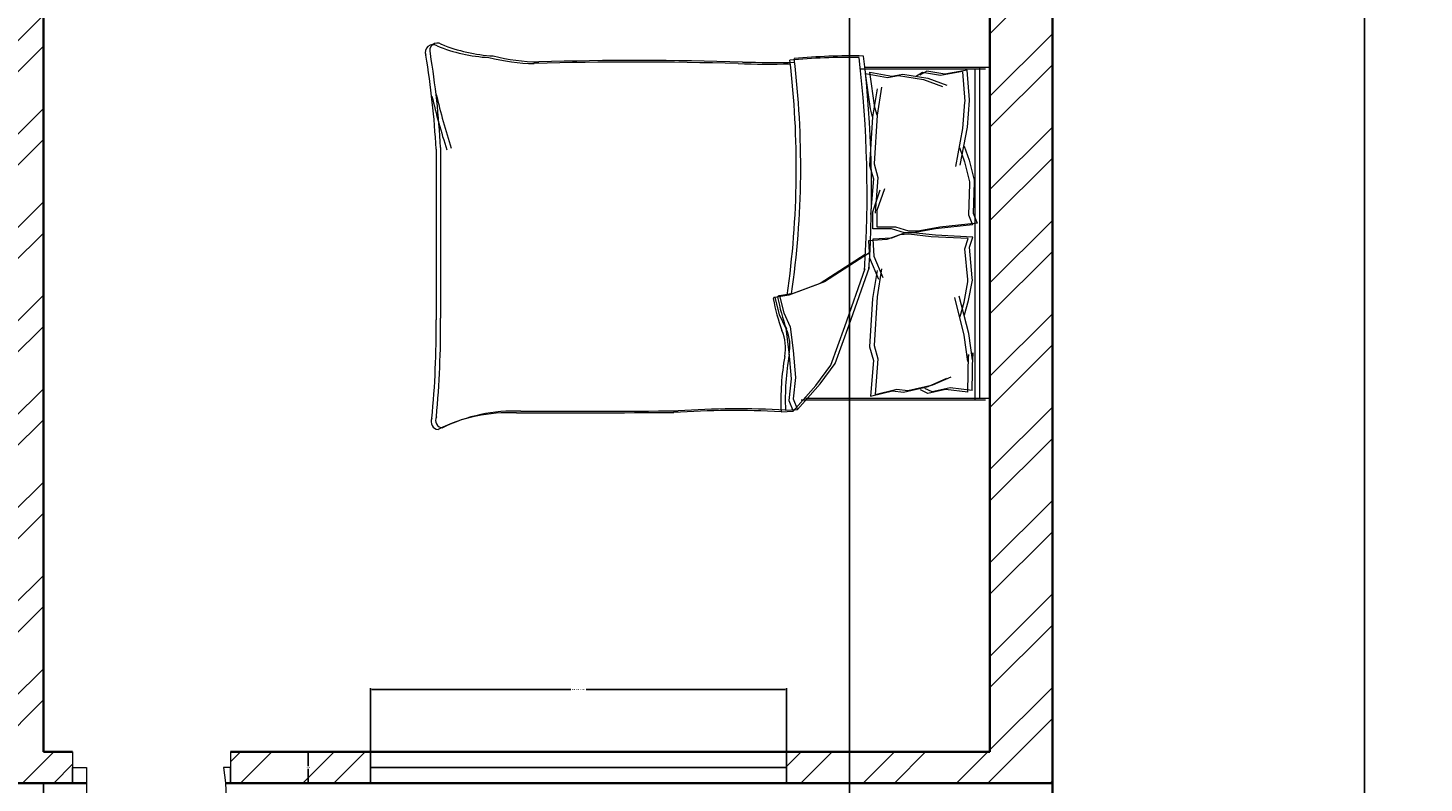
# Model space of a CAD drawing. Units: inches. Extents: x 2120 to 4013, y 1390 to 3019.
# Tile 21 of 59: x 2862 to 3063, y 1582 to 1690. Entities that reach past the tile are written whole.
import ezdxf

# ---------------------------------------------------------------- set-up
doc = ezdxf.new("R2010")
doc.units = ezdxf.units.IN
for name, color, linetype, lineweight in [('A-ANNO-DIMS', 2, 'Continuous', 18), ('A-DOOR', 3, 'Continuous', 18), ('A-FLOR-DECK', 7, 'Continuous', 25), ('A-FURN', 8, 'Continuous', 13), ('A-GLAZ', 4, 'Continuous', 18), ('A-WALL', 7, 'Continuous', 35), ('A-WALL-PATT', 252, 'Continuous', 13)]:
    doc.layers.add(name, color=color, linetype=linetype, lineweight=lineweight)
doc.styles.get("Standard").update_dxf_attribs({"font": 'arial.ttf'})
doc.dimstyles.get("Standard").update_dxf_attribs({"dimtxt": 0.18, "dimasz": 0.18, "dimexe": 0.18, "dimexo": 0.0625, "dimgap": 0.09, "dimtad": 0, "dimtih": 1, "dimtoh": 1, "dimdec": 4, "dimzin": 0, "dimdsep": 46, "dimtxsty": 'Standard', "dimcen": 0.09, "dimadec": 0, "dimazin": 0, "dimtfac": 1, "dimtdec": 4, "dimtofl": 0, "dimtmove": 0, "dimatfit": 3, "dimfxl": 1, "dimtolj": 1, "dimtzin": 0, "dimarcsym": 0})

# ---------------------------------------------------------------- blocks, each defined once
blk = doc.blocks.new('BED-DOUBLE-PLAN')
for p, q in [((3.48, 63.34), (3.48, 81.45)), ((3.48, 81.45), (51.27, 81.45)), ((3.7, 62.7), (3.7, 80.81)), ((51.27, 81.45), (51.27, 54.84)), ((51.5, 80.81), (51.5, 54.2)), ((3.48, 79.91), (51.27, 79.91)), ((3.7, 79.27), (51.5, 79.27)), ((16.88, 78.42), (19.77, 79.14)), ((19.77, 79.14), (20.09, 79.14)), ((20.09, 79.14), (24.54, 79)), ((24.54, 79), (25.98, 79.58)), ((24.77, 78.36), (26.21, 78.94)), ((25.98, 79.58), (26.56, 74.23)), ((26.21, 78.94), (26.79, 73.59)), ((27.98, 78.95), (27.73, 73.58)), ((29.46, 78.47), (27.98, 78.95)), ((33.89, 78.89), (29.46, 78.47)), ((34.21, 78.91), (33.89, 78.89)), ((37.14, 78.37), (34.21, 78.91)), ((45.71, 78.9), (41.92, 78.38)), ((50.11, 78.89), (44.71, 78.99)), ((44.71, 78.99), (45.71, 78.9)), ((50.11, 78.89), (49.73, 75.68)), ((3.9, 78.11), (8.18, 78.44)), ((3.9, 78.13), (4.47, 74.95)), ((4.12, 77.49), (4.7, 74.31)), ((4.13, 77.47), (8.41, 77.8)), ((8.18, 78.44), (8.29, 78.42)), ((8.29, 78.42), (12.11, 78.13)), ((8.41, 77.8), (8.51, 77.78)), ((8.51, 77.78), (12.34, 77.49)), ((12.11, 78.13), (17.6, 77.12)), ((12.34, 77.49), (17.83, 76.48)), ((14.86, 77.7), (16.88, 78.42)), ((15.08, 77.06), (17.11, 77.78)), ((17.11, 77.78), (20, 78.5)), ((20, 78.5), (20.32, 78.5)), ((20.32, 78.5), (24.77, 78.36)), ((28.21, 78.32), (27.96, 72.94)), ((29.69, 77.83), (28.21, 78.32)), ((34.11, 78.25), (29.69, 77.83)), ((34.43, 78.27), (34.11, 78.25)), ((37.37, 77.73), (34.43, 78.27)), ((41.92, 78.38), (36.5, 77.02)), ((42.14, 77.74), (36.72, 76.38)), ((39.2, 77.77), (37.14, 78.37)), ((39.43, 77.13), (37.37, 77.73)), ((45.94, 78.26), (42.14, 77.74)), ((50.34, 78.25), (44.94, 78.35)), ((44.94, 78.35), (45.94, 78.26)), ((50.34, 78.25), (49.96, 75.04)), ((4.47, 74.95), (4.04, 72.35)), ((5.05, 72.49), (6.06, 75.24)), ((5.28, 71.85), (6.29, 74.6)), ((49.31, 73.19), (48.13, 75.87)), ((49.54, 72.55), (48.36, 75.23)), ((49.73, 75.68), (50.33, 73.11)), ((49.96, 75.04), (50.56, 72.47)), ((4.7, 74.31), (4.27, 71.71)), ((4.47, 68.88), (5.05, 72.49)), ((26.56, 74.23), (27.14, 71.05)), ((26.79, 73.59), (27.37, 70.41)), ((27.73, 73.58), (27.36, 70.37)), ((27.96, 72.94), (27.58, 69.73)), ((50.11, 69.62), (49.31, 73.19)), ((50.34, 68.98), (49.54, 72.55)), ((50.33, 73.11), (49.82, 72.06)), ((4.04, 72.35), (4.62, 71.33)), ((4.27, 71.71), (4.85, 70.7)), ((4.7, 68.24), (5.28, 71.85)), ((27.14, 71.05), (27.14, 69.74)), ((50.56, 72.47), (50.04, 71.42)), ((4.76, 67.29), (4.47, 68.88)), ((27.14, 69.74), (26.56, 67.86)), ((27.37, 69.1), (26.79, 67.23)), ((27.36, 70.37), (27.44, 69.07)), ((27.37, 70.41), (27.37, 69.1)), ((27.44, 69.07), (28.13, 67.23)), ((27.58, 69.73), (27.67, 68.43)), ((49.92, 68.01), (50.11, 69.62)), ((50.15, 67.37), (50.34, 68.98)), ((4.19, 64.11), (4.76, 67.29)), ((4.41, 63.47), (4.99, 66.65)), ((4.99, 66.65), (4.7, 68.24)), ((26.56, 67.86), (26.56, 65.18)), ((26.79, 67.23), (26.79, 64.54)), ((27.67, 68.43), (28.36, 66.59)), ((28.13, 67.23), (28.3, 64.55)), ((28.36, 66.59), (28.53, 63.91)), ((50.7, 64.87), (49.92, 68.01)), ((50.93, 64.23), (50.15, 67.37)), ((9.28, 64.83), (4.19, 64.11)), ((6.38, 65.82), (10.42, 65.15)), ((6.61, 65.18), (10.64, 64.51)), ((10.42, 65.15), (9.28, 64.83)), ((10.64, 64.51), (9.51, 64.19)), ((10.42, 65.15), (17.43, 64.72)), ((10.64, 64.51), (17.65, 64.08)), ((17.43, 64.72), (19.39, 65.28)), ((17.65, 64.08), (19.61, 64.64)), ((19.39, 65.28), (24.52, 64.87)), ((19.61, 64.64), (24.75, 64.23)), ((24.1, 65.18), (20.96, 66.27)), ((24.33, 64.54), (21.19, 65.63)), ((26.56, 65.18), (24.1, 65.18)), ((26.79, 64.54), (24.33, 64.54)), ((28.3, 64.55), (30.75, 64.71)), ((30.75, 64.71), (33.82, 65.99)), ((30.98, 64.07), (34.05, 65.35)), ((32.57, 65.82), (36.6, 65.15)), ((32.79, 65.18), (36.83, 64.51)), ((36.6, 65.15), (43.61, 64.72)), ((36.83, 64.51), (43.84, 64.08)), ((43.61, 64.72), (45.57, 65.28)), ((43.84, 64.08), (45.8, 64.64)), ((45.57, 65.28), (50.7, 64.87)), ((45.8, 64.64), (50.93, 64.23)), ((9.51, 64.19), (4.41, 63.47)), ((28.53, 63.91), (30.98, 64.07)), ((30.26, 64.06), (34.45, 57.57)), ((30.49, 63.42), (34.68, 56.93)), ((40.65, 61.13), (32.31, 64.06)), ((40.87, 60.49), (32.54, 63.42)), ((46.22, 59.12), (40.65, 61.13)), ((46.45, 58.48), (40.87, 60.49)), ((49.16, 56.95), (46.22, 59.12)), ((49.39, 56.31), (46.45, 58.48)), ((34.45, 57.57), (36.15, 53.08)), ((34.68, 56.93), (36.38, 52.44)), ((52.87, 53.7), (49.16, 56.95)), ((53.1, 53.06), (49.39, 56.31)), ((36.15, 53.08), (36.46, 51.07)), ((36.38, 52.44), (36.69, 50.43)), ((38.94, 51.69), (40.96, 52.62)), ((40.96, 52.62), (44.36, 53.08)), ((41.18, 51.98), (44.59, 52.44)), ((44.36, 53.08), (48.23, 53.39)), ((44.59, 52.44), (48.46, 52.75)), ((48.23, 53.39), (51.33, 53.08)), ((48.46, 52.75), (51.56, 52.44)), ((51.33, 53.08), (52.87, 53.7)), ((51.56, 52.44), (53.1, 53.06)), ((52.95, 51.96), (52.87, 53.7, 3.87)), ((53.18, 51.32), (53.1, 53.06, 3.87)), ((36.46, 51.07), (38.94, 51.69)), ((36.69, 50.43), (39.17, 51.05)), ((39.17, 51.05), (41.18, 51.98)), ((15.06, 2.2), (39.68, 2.2)), ((15.29, 1.56), (39.91, 1.56))]:
    blk.add_line(p, q)
for centre, radius, start, end in [((85.16, 61.35), 83.31, 178.7218, 185.604), ((21.36, -100.61), 164.97, 86.0865, 96.7821), ((85.39, 60.71), 83.31, 178.7218, 185.604), ((21.59, -101.25), 164.97, 86.0865, 96.7821), ((17.76, -74.87), 129.02, 81.7845, 96.9006), ((17.99, -75.51), 129.02, 81.7845, 96.9006), ((-167.31, 50.27), 170.11, 358.4762, 1.0082), ((-167.08, 49.63), 170.11, 358.4762, 1.0082), ((43.74, 46.38), 6.22, 78.6608, 113.7384), ((51.33, 88.1), 36.18, 259.8763, 272.5657), ((36.64, 51.01), 0.185, 160.2464, 271.1377), ((31.16, 79.96), 29.65, 280.6617, 289.8806), ((36.87, 50.37), 0.185, 160.2464, 271.1377), ((31.38, 79.32), 29.65, 280.6617, 289.8806), ((43.97, 45.74), 6.22, 78.6608, 113.7384), ((51.56, 87.46), 36.18, 259.8763, 272.5657), ((182.27, 45.13), 129.5, 176.9791, 183.8365), ((182.5, 44.49), 129.5, 176.9791, 183.8365), ((484.82, 30.83), 482.31, 178.2277, 181.7185), ((485.05, 30.19), 482.31, 178.2277, 181.7185), ((-4508.74, 13.62), 4561.86, 0.00217, 0.28689), ((-4508.51, 12.99), 4561.86, 0.00217, 0.28689), ((-26.9, 16.93), 29.63, 346.0648, 358.9113), ((-26.67, 16.29), 29.63, 346.0648, 358.9113), ((76.16, 12.78), 23.07, 177.4714, 206.4681), ((76.39, 12.14), 23.07, 177.4714, 206.4681), ((-21.66, 11.17), 23.56, 337.9751, 356.652), ((-21.43, 10.53), 23.56, 337.9751, 356.652), ((1.09, 1.73), 1.09, 146.1736, 293.4781), ((21.43, -119.39), 121.76, 92.9958, 99.4091), ((-17.22, 105.16), 106.46, 283.3832, 287.7053), ((-16.99, 104.52), 106.46, 283.3832, 287.7053), ((41.15, -130.83), 133.04, 84.4998, 90.6351), ((54.41, 2.58), 1.1, 242.6588, 356.02), ((1.32, 1.09), 1.09, 146.1736, 293.4781), ((21.66, -120.03), 121.76, 92.9958, 99.4091), ((41.38, -131.47), 133.04, 84.4998, 90.6351), ((54.64, 1.94), 1.1, 242.6588, 356.02)]:
    blk.add_arc(centre, radius, start, end)
blk = doc.blocks.new('DOOR-SWING-24IN-100p95DEG')
for p, q in [((0, 26.25), (0, 21.75)), ((22.8, 26.25), (22.8, 21.75)), ((0, 21.75), (0, 24)), ((0, 24), (2, 24)), ((2, 24), (2, 0)), ((22.8, 24), (21.8, 24)), ((22.8, 21.75), (22.8, 24))]:
    blk.add_line(p, q)
blk.add_arc((2, 20.17), 20.17, 270, 10.9508)
blk = doc.blocks.new('WIN-PLAN-60IN-03')
for p, q in [((0, 4.5), (0, 0)), ((60, 2.25), (60, 4.5)), ((60, 4.5), (60, 0)), ((0, 0), (0, 2.25)), ((0, 2.25), (60, 2.25))]:
    blk.add_line(p, q)
blk = doc.blocks.new('*D187')
at = {"layer": 'A-ANNO-DIMS', "color": 0, "lineweight": -2, "transparency": 16777216}
for p, q in [((2911.39, 1586.09), (2911.39, 1595.21)), ((2911.57, 1595.03), (2940.27, 1595.03)), ((2971.21, 1595.03), (2942.51, 1595.03)), ((2971.39, 1586.09), (2971.39, 1595.21))]:
    blk.add_line(p, q, dxfattribs=at)
at = {"layer": 'A-ANNO-DIMS', "color": 0, "transparency": 16777216}
for points in [[(2911.57, 1595.06), (2911.57, 1595), (2911.39, 1595.03)], [(2971.21, 1595.06), (2971.21, 1595), (2971.39, 1595.03)]]:
    blk.add_solid(points, dxfattribs=at)
at = {"layer": 'Defpoints', "color": 0, "transparency": 16777216}
for p in [(2971.39, 1595.03), (2911.39, 1586.03), (2971.39, 1586.03)]:
    blk.add_point(p, dxfattribs=at)
at = {"layer": 'A-ANNO-DIMS', "color": 0, "transparency": 16777216, "insert": (2941.39, 1595.03), "char_height": 0.18, "attachment_point": 5}
blk.add_mtext('\\A1;WINDOW 60 TYP.', dxfattribs=at)
blk = doc.blocks.new('*D188')
at = {"layer": 'A-ANNO-DIMS', "color": 0, "lineweight": -2, "transparency": 16777216}
for p, q in [((2911.33, 1586.03), (2902.21, 1586.03)), ((2902.39, 1585.85), (2902.39, 1583.96)), ((2902.39, 1581.71), (2902.39, 1583.6)), ((2911.33, 1581.53), (2902.21, 1581.53))]:
    blk.add_line(p, q, dxfattribs=at)
at = {"layer": 'A-ANNO-DIMS', "color": 0, "transparency": 16777216}
for points in [[(2902.36, 1585.85), (2902.42, 1585.85), (2902.39, 1586.03)], [(2902.36, 1581.71), (2902.42, 1581.71), (2902.39, 1581.53)]]:
    blk.add_solid(points, dxfattribs=at)
at = {"layer": 'Defpoints', "color": 0, "transparency": 16777216}
for p in [(2902.39, 1586.03), (2911.39, 1586.03), (2911.39, 1581.53)]:
    blk.add_point(p, dxfattribs=at)
at = {"layer": 'A-ANNO-DIMS', "color": 0, "transparency": 16777216, "insert": (2902.39, 1583.78), "char_height": 0.18, "attachment_point": 5}
blk.add_mtext('\\A1;5 TYP.', dxfattribs=at)
blk = doc.blocks.new('*D212')
at = {"layer": 'A-ANNO-DIMS', "color": 0, "lineweight": -2, "transparency": 16777216}
for p, q in [((3009.8, 2352.53), (3054.91, 2352.53)), ((3054.73, 2352.35), (3054.73, 1947.71)), ((3054.73, 1542.71), (3054.73, 1947.35)), ((3009.8, 1542.53), (3054.91, 1542.53))]:
    blk.add_line(p, q, dxfattribs=at)
at = {"layer": 'A-ANNO-DIMS', "color": 0, "transparency": 16777216}
for points in [[(3054.7, 2352.35), (3054.76, 2352.35), (3054.73, 2352.53)], [(3054.7, 1542.71), (3054.76, 1542.71), (3054.73, 1542.53)]]:
    blk.add_solid(points, dxfattribs=at)
at = {"layer": 'Defpoints', "color": 0, "transparency": 16777216}
for p in [(3009.73, 2352.53), (3009.73, 1542.53), (3054.73, 1542.53)]:
    blk.add_point(p, dxfattribs=at)
at = {"layer": 'A-ANNO-DIMS', "color": 0, "transparency": 16777216, "insert": (3054.73, 1947.53), "char_height": 0.18, "attachment_point": 5}
blk.add_mtext('\\A1;810', dxfattribs=at)
blk = doc.blocks.new('*D217')
at = {"layer": 'A-ANNO-DIMS', "color": 0, "lineweight": -2, "transparency": 16777216}
for p, q in [((3071.67, 2352.53), (2980.31, 2352.53)), ((2980.49, 2352.35), (2980.49, 1947.71)), ((2980.49, 1542.71), (2980.49, 1947.35)), ((3305.67, 1542.53), (2980.31, 1542.53))]:
    blk.add_line(p, q, dxfattribs=at)
at = {"layer": 'A-ANNO-DIMS', "color": 0, "transparency": 16777216}
for points in [[(2980.46, 2352.35), (2980.52, 2352.35), (2980.49, 2352.53)], [(2980.46, 1542.71), (2980.52, 1542.71), (2980.49, 1542.53)]]:
    blk.add_solid(points, dxfattribs=at)
at = {"layer": 'Defpoints', "color": 0, "transparency": 16777216}
for p in [(2980.49, 2352.53), (3071.73, 2352.53), (3305.73, 1542.53)]:
    blk.add_point(p, dxfattribs=at)
at = {"layer": 'A-ANNO-DIMS', "color": 0, "transparency": 16777216, "insert": (2980.49, 1947.53), "char_height": 0.18, "attachment_point": 5}
blk.add_mtext('\\A1;810', dxfattribs=at)

msp = doc.modelspace()

# ---------------------------------------------------------------- hatches: boundary and pattern name
at = {"layer": 'A-WALL-PATT'}
h = msp.add_hatch(dxfattribs=at)
h.set_pattern_fill('ANSI32', color=256)
h.paths.add_polyline_path([(2271.7331, 2122.6377), (2262.7331, 2122.6377), (2262.7331, 2040.3893), (2267.2331, 2040.3893), (2271.7331, 2040.3893), (2271.7331, 2044.8856), (2271.7331, 2070.531), (2391.7331, 2070.531), (2391.7331, 1926.5306), (2388.3993, 1926.5306), (2388.3993, 1922.531), (2395.7331, 1922.531), (2395.7331, 1992.531), (2400.4511, 1992.531), (2400.4511, 1997.0306), (2395.7331, 1997.0306), (2395.7331, 2070.531), (2443.7331, 2070.531), (2443.7331, 2046.1368), (2448.2331, 2046.1368), (2448.2331, 2070.531), (2580.2331, 2070.531), (2580.2331, 1997.0306), (2492.9076, 1997.0306), (2492.9076, 1992.531), (2580.2331, 1992.531), (2580.2331, 1983.9368), (2589.2331, 1983.9368), (2589.2331, 2070.531), (2589.2331, 2075.0306), (2396.2331, 2075.0306), (2396.2331, 2184.3565), (2393.9831, 2184.3565), (2391.7331, 2184.3565), (2391.7331, 2075.0306), (2271.7331, 2075.0306)])
h.paths.add_polyline_path([(2724.7331, 2138.0306), (2628.7331, 2138.0306), (2628.7331, 2070.5306), (2628.7331, 2067.0987), (2633.2331, 2067.0987), (2637.7331, 2067.0987), (2637.7331, 2070.531), (2657.3413, 2070.531), (2657.3413, 2079.5306), (2637.7331, 2079.5306), (2637.7331, 2129.031), (2715.7331, 2129.031), (2715.7331, 2079.5306), (2698.0378, 2079.5306), (2698.0378, 2070.531), (2715.7331, 2070.531), (2715.7331, 2012.1531), (2720.2331, 2012.1531), (2724.7331, 2012.1531)])
h.paths.add_polyline_path([(2724.7331, 2213.031), (2831.3209, 2213.031), (2831.3209, 2215.281), (2831.3209, 2217.5306), (2724.7331, 2217.5306), (2724.7331, 2343.531), (2751.8755, 2343.531), (2751.8755, 2352.5306), (2715.7331, 2352.5306), (2715.7331, 2138.031), (2724.7331, 2138.031)])
h.paths.add_polyline_path([(2902.53, 2352.5306), (2811.8755, 2352.5306), (2811.8755, 2343.531), (2867.2331, 2343.531), (2867.2331, 2217.5306), (2863.6364, 2217.5306), (2863.6364, 2213.031), (2871.7331, 2213.031), (2871.7331, 2217.531), (2871.7331, 2343.531), (2902.53, 2343.531)])
h.paths.add_polyline_path([(3009.7331, 2352.5306), (2938.53, 2352.5306), (2938.53, 2343.531), (2966.2331, 2343.531), (2966.2331, 2242.3281), (2968.4831, 2242.3281), (2970.7331, 2242.3281), (2970.7331, 2343.531), (3009.7331, 2343.531)])
h.paths.add_polyline_path([(3009.7331, 2217.5306), (2970.7331, 2217.5306), (2970.7331, 2220.5422), (2968.4831, 2220.5422), (2966.2331, 2220.5422), (2966.2331, 2217.5306), (2911.7752, 2217.5306), (2907.7331, 2217.5306), (2907.7331, 2213.0306), (2907.7331, 2194.9663), (2912.2331, 2194.9663), (2912.2331, 2213.031), (2970.7331, 2213.031), (3000.7331, 2213.031), (3000.7331, 2205.523), (3009.7331, 2205.523)])
h.paths.add_polyline_path([(3009.7331, 2181.5227), (3000.7331, 2181.5227), (3000.7331, 2165.0306), (2912.2331, 2165.0306), (2912.2331, 2170.8202), (2907.7331, 2170.8202), (2907.7331, 2165.0306), (2899.5169, 2165.0306), (2899.5169, 2162.7806), (2899.5169, 2160.531), (2907.7331, 2160.531), (2907.7331, 2137.3432), (2912.2331, 2137.3432), (2912.2331, 2160.531), (3000.7331, 2160.531), (3000.7331, 2150.4993), (3009.7331, 2150.4993)])
h.paths.add_polyline_path([(3009.7331, 2126.499), (3005.2331, 2126.499), (3000.7331, 2126.499), (3000.7331, 2112.5306), (2912.2331, 2112.5306), (2912.2331, 2115.6036), (2907.7331, 2115.6036), (2907.7331, 2108.031), (3000.7331, 2108.031), (3000.7331, 2084.7256), (3009.7331, 2084.7256)], flags=17)
h.paths.add_polyline_path([(3009.7331, 1971.531), (3009.7331, 2024.7253), (3000.7331, 2024.7253), (3000.7331, 2006.4153), (3000.7331, 1971.5306), (2864.2331, 1971.5306), (2864.2331, 2160.531), (2868.0522, 2160.531), (2868.0522, 2165.0306), (2859.7331, 2165.0306), (2859.7331, 1971.5306), (2724.7331, 1971.5306), (2724.7331, 1977.7012), (2715.7331, 1977.7012), (2715.7331, 1962.5306), (2715.7331, 1950.9035), (2720.2331, 1950.9035), (2724.7331, 1950.9035), (2724.7331, 1962.531), (2855.2331, 1962.531), (2859.7331, 1962.531), (2859.7331, 1835.031), (2864.2331, 1834.8158), (2864.2331, 1962.531), (2958.7331, 1962.531), (2958.7331, 1937.0925), (2963.2331, 1937.0925), (2963.2331, 1962.531), (3000.7331, 1962.531), (3009.7331, 1962.531)])
h.paths.add_polyline_path([(2724.7331, 1728.531), (2822.7164, 1728.531), (2822.7164, 1733.0306), (2724.7331, 1733.0306), (2724.7331, 1779.3416), (2715.7331, 1779.3416), (2715.7331, 1581.531), (2753.02, 1581.531), (2753.02, 1586.031), (2753.02, 1590.5306), (2724.7331, 1590.5306)])
h.paths.add_polyline_path([(2864.2331, 1590.531), (2864.2331, 1787.031), (2868.4075, 1787.031), (2868.4075, 1791.5306), (2859.7331, 1791.5306), (2859.7331, 1739.0306), (2859.7331, 1733.0306), (2854.3125, 1733.0306), (2854.3125, 1728.531), (2859.7331, 1728.531), (2859.7331, 1590.5306), (2813.02, 1590.5306), (2813.02, 1581.531), (2868.4123, 1581.531), (2868.4123, 1583.781), (2868.4123, 1586.0306), (2864.2331, 1586.0306)])
h.paths.add_polyline_path([(3009.7331, 1754.6619), (3000.7331, 1754.6619), (3000.7331, 1739.0306), (2912.2331, 1739.0306), (2912.2331, 1742.2257), (2907.7331, 1742.2257), (2907.7331, 1739.0306), (2907.7331, 1734.531), (3000.7331, 1734.531), (3000.7331, 1590.5306), (3000.7331, 1586.0306), (2971.3921, 1586.0306), (2971.3921, 1581.531), (3009.7331, 1581.531)])
h.paths.add_polyline_path([(2911.3921, 1583.781), (2911.3921, 1586.0306), (2891.2138, 1586.0306), (2891.2138, 1581.531), (2911.3921, 1581.531)])
h.paths.add_polyline_path([(3009.7331, 1799.8422), (3000.7331, 1799.8422), (3000.7331, 1791.5306), (2912.2331, 1791.5306), (2912.2331, 1796.3264), (2909.9831, 1796.3264), (2907.7331, 1796.3264), (2907.7331, 1791.5306), (2902.7033, 1791.5306), (2902.7033, 1787.031), (2907.7331, 1787.031), (2907.7331, 1761.1622), (2912.2331, 1761.1622), (2912.2331, 1787.031), (3000.7331, 1787.031), (3000.7331, 1778.6622), (3009.7331, 1778.6622)])
h.paths.add_polyline_path([(3009.7331, 1839.5306), (2963.2331, 1839.5306), (2963.2331, 1842.8629), (2960.9831, 1842.8629), (2958.7331, 1842.8629), (2958.7331, 1839.5306), (2907.7331, 1839.5306), (2907.7331, 1814.4599), (2912.2331, 1814.4599), (2912.2331, 1835.031), (3000.7331, 1835.031), (3000.7331, 1823.8425), (3009.7331, 1823.8425), (3009.7331, 1835.031)])
h.paths.add_polyline_path([(2963.2331, 1901.0922), (2960.9831, 1901.0922), (2958.7331, 1901.0922), (2958.7331, 1862.8843), (2963.2331, 1862.8843)], flags=17)
h.paths.add_polyline_path([(2724.7331, 1891.9826), (2724.7331, 1914.3416), (2715.7331, 1914.3416), (2715.7331, 1783.8416), (2637.7331, 1783.8416), (2637.7331, 1914.3416), (2628.7331, 1914.3416), (2624.7701, 1914.3416), (2624.7701, 1909.8416), (2624.7701, 1905.3419), (2628.7331, 1905.3419), (2628.7331, 1876.9915), (2628.7331, 1779.3419), (2637.7331, 1779.3419), (2715.7331, 1779.3419), (2724.7331, 1779.3419), (2724.7331, 1835.031)])
h.paths.add_polyline_path([(2637.7331, 1731.531), (2637.7331, 1779.3416), (2628.7331, 1779.3416), (2628.7331, 1731.5306), (2589.2331, 1731.5306), (2535.9814, 1731.5306), (2496.7331, 1731.5306), (2496.7331, 1725.6876), (2498.9831, 1725.6876), (2501.2331, 1725.6876), (2501.2331, 1727.031), (2628.7331, 1727.031), (2628.7331, 1680.4203), (2628.7331, 1590.5306), (2628.7331, 1586.0306), (2604.1361, 1586.0306), (2604.1361, 1581.531), (2637.7331, 1581.531), (2637.7331, 1590.531)])

# ---------------------------------------------------------------- linework, layer by layer
at = {"layer": 'A-FLOR-DECK'}
for p, q in [((2864.2331, 1542.531), (2864.2331, 1581.531)), ((2864.2331, 1542.5306), (2864.2331, 1581.5306))]:
    msp.add_line(p, q, dxfattribs=at)
at = {"layer": 'A-WALL'}
for p, q in [((3009.7331, 1962.531), (3009.7331, 1542.531)), ((3009.7331, 1962.5306), (3009.7331, 1542.5306)), ((2864.2331, 1590.531), (2864.2331, 1787.031)), ((2864.2331, 1590.5306), (2864.2331, 1787.0306)), ((3000.7331, 1734.531), (3000.7331, 1590.531)), ((3000.7331, 1734.531), (3000.7331, 1586.031)), ((3000.7331, 1734.5306), (3000.7331, 1586.0306)), ((3000.7331, 1734.5306), (3000.7331, 1590.5306)), ((2864.2331, 1590.531), (2864.2331, 1586.031)), ((2864.2331, 1590.5306), (2864.2331, 1586.0306)), ((2868.4123, 1586.031), (2864.2331, 1586.031)), ((2868.4124, 1586.0306), (2864.2331, 1586.0306)), ((3000.7331, 1586.031), (2891.2137, 1586.031)), ((3000.7331, 1586.0306), (2891.2138, 1586.0306)), ((2870.4123, 1581.531), (2715.7331, 1581.531)), ((2870.4124, 1581.5306), (2715.7331, 1581.5306)), ((3009.7331, 1581.531), (2890.5189, 1581.531)), ((3009.7331, 1581.5306), (2890.5189, 1581.5306))]:
    msp.add_line(p, q, dxfattribs=at)

# ---------------------------------------------------------------- block references
at = {"layer": 'A-DOOR'}
for p in [(2868.4123, 1559.781), (2868.4124, 1559.7806)]:
    msp.add_blockref('DOOR-SWING-24IN-100p95DEG', p, dxfattribs=at)
at = {"layer": 'A-FURN'}
for p, rotation in [((2919.2869, 1688.2853), 270.0000000000001), ((2919.2869, 1688.285), 270)]:
    msp.add_blockref('BED-DOUBLE-PLAN', p, dxfattribs=dict(at, rotation=rotation))
at = {"layer": 'A-GLAZ'}
msp.add_blockref('WIN-PLAN-60IN-03', (2911.3921, 1581.531), dxfattribs=at)
at = {"layer": 'A-GLAZ', "rotation": 180}
msp.add_blockref('WIN-PLAN-60IN-03', (2971.3921, 1586.0306), dxfattribs=at)

# ---------------------------------------------------------------- dimensions: what is measured, and where the dimension line sits
at = {"layer": 'A-ANNO-DIMS'}
for base, p1, p2, picture, middle in [((2980.4877, 2352.531), (3305.7347, 1542.531), (3071.7347, 2352.531), '*D217', (2980.4877, 1947.531)), ((3054.7331, 1542.531), (3009.7331, 2352.531), (3009.7331, 1542.531), '*D212', (3054.7331, 1947.531))]:
    dim = msp.add_linear_dim(base=base, p1=p1, p2=p2, angle=90, dimstyle='Standard', override={"dimdec": 0, "dimlfac": 1, "dimrnd": 0, "dimzin": 0, "dimdsep": 46, "dimlunit": 2}, dxfattribs=at)
    dim.commit()
    dim.dimension.update_dxf_attribs({"geometry": picture, "text_midpoint": middle})
dim = msp.add_linear_dim(base=(2971.3921, 1595.031), p1=(2911.3921, 1586.031), p2=(2971.3921, 1586.031), text='WINDOW <> TYP.', dimstyle='Standard', override={"dimdec": 0, "dimlfac": 1, "dimrnd": 0, "dimzin": 0, "dimdsep": 46, "dimlunit": 2}, dxfattribs=at)
dim.commit()
dim.dimension.update_dxf_attribs({"geometry": '*D187', "text_midpoint": (2941.3921, 1595.031)})
dim = msp.add_linear_dim(base=(2902.3921146522, 1586.03095126), p1=(2911.3921146522, 1581.53095126), p2=(2911.3921146522, 1586.03095126), angle=90, text='<> TYP.', dimstyle='Standard', override={"dimdec": 0, "dimlfac": 1, "dimrnd": 0, "dimzin": 0, "dimdsep": 46, "dimlunit": 2}, dxfattribs=at)
dim.commit()
dim.dimension.update_dxf_attribs({"geometry": '*D188', "text_midpoint": (2902.3921146522, 1583.78095126)})

doc.saveas('drawing.dxf')
